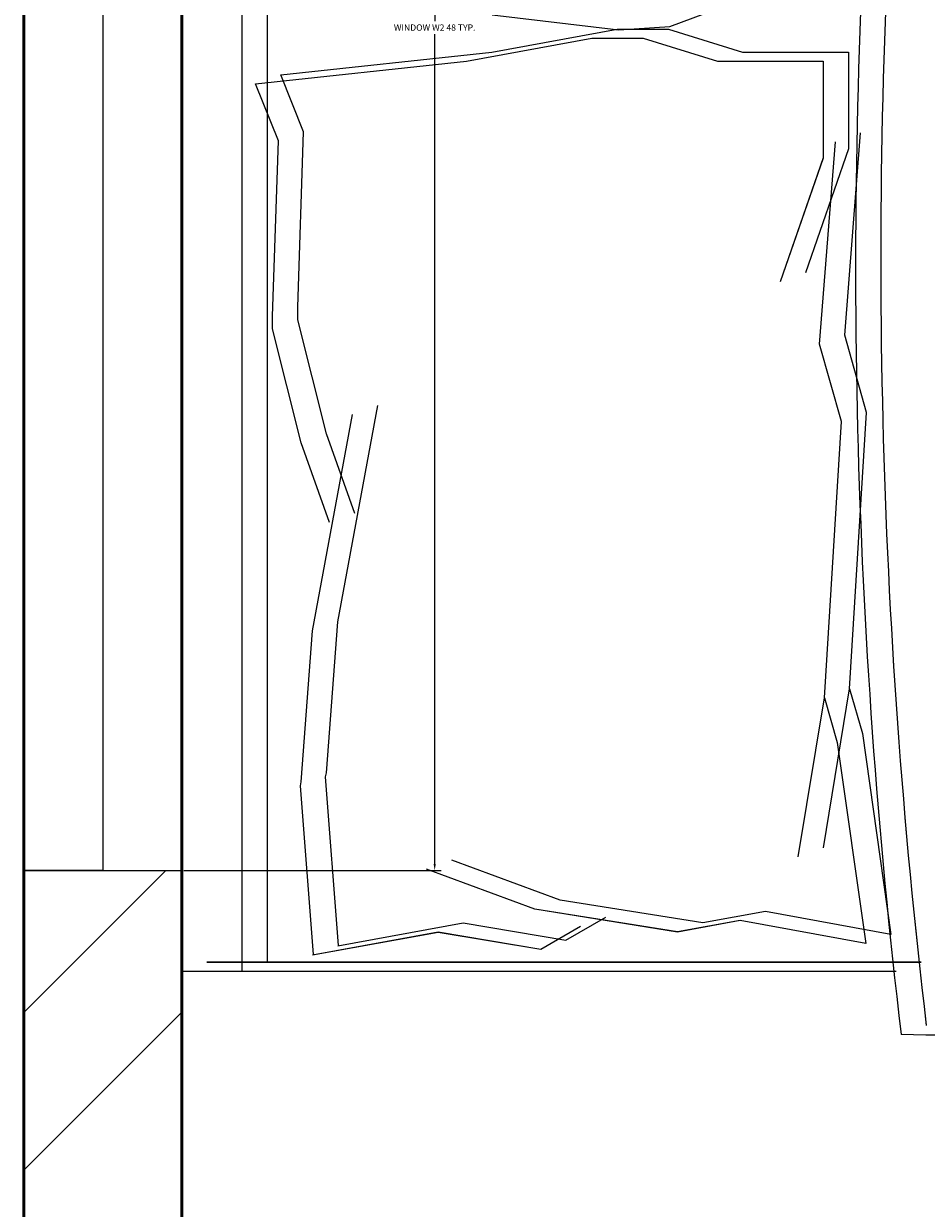
# Model space of a CAD drawing. Units: inches. Extents: x 1901 to 2863, y 888 to 2433.
# Tile 55 of 91: x 2025 to 2051, y 2127 to 2161. Entities that reach past the tile are written whole.
import ezdxf

# ---------------------------------------------------------------- set-up
doc = ezdxf.new("R2010")
doc.units = ezdxf.units.IN
for name, color, linetype, lineweight in [('A-ANNO-DIMS', 2, 'Continuous', 18), ('A-FURN', 8, 'Continuous', 18), ('A-GLAZ', 3, 'Continuous', 25), ('A-WALL', 7, 'Continuous', 50), ('A-WALL-PATT', 8, 'Continuous', 13)]:
    doc.layers.add(name, color=color, linetype=linetype, lineweight=lineweight)
doc.styles.get("Standard").update_dxf_attribs({"font": 'arial.ttf'})
doc.dimstyles.get("Standard").update_dxf_attribs({"dimtxt": 0.18, "dimasz": 0.18, "dimexe": 0.18, "dimexo": 0.0625, "dimgap": 0.09, "dimtad": 0, "dimtih": 1, "dimtoh": 1, "dimdec": 4, "dimzin": 0, "dimdsep": 46, "dimtxsty": 'Standard', "dimcen": 0.09, "dimadec": 0, "dimazin": 0, "dimtfac": 1, "dimtdec": 4, "dimtofl": 0, "dimtmove": 0, "dimatfit": 3, "dimfxl": 1, "dimtolj": 1, "dimtzin": 0, "dimarcsym": 0})

# ---------------------------------------------------------------- blocks, each defined once
blk = doc.blocks.new('BED-DOUBLE')
for p, q in [((0.026, 57.778), (0.026, 4.122)), ((13.922, 30.767), (15.988, 31.547)), ((13.922, 30.767), (15.988, 31.547)), ((8.859, 31.101), (12.464, 30.676)), ((8.859, 31.101), (12.464, 30.676)), ((12.464, 30.676), (13.922, 30.767)), ((12.464, 30.676), (13.922, 30.767)), ((8.132, 29.785), (11.704, 30.434)), ((8.132, 29.784), (11.704, 30.434)), ((8.85, 30.041), (12.422, 30.69)), ((8.85, 30.041), (12.422, 30.69)), ((11.704, 30.434), (13.165, 30.434)), ((11.704, 30.434), (13.165, 30.434)), ((12.422, 30.69), (13.883, 30.69)), ((12.422, 30.69), (13.883, 30.69)), ((13.165, 30.434), (15.275, 29.785)), ((13.165, 30.434), (15.275, 29.784)), ((13.883, 30.69), (15.993, 30.041)), ((13.883, 30.69), (15.993, 30.041)), ((2.844, 29.392), (8.85, 30.041)), ((2.844, 29.392), (8.85, 30.041)), ((15.993, 30.041), (19.003, 30.041)), ((15.993, 30.041), (19.003, 30.041)), ((19.003, 30.041), (19.003, 27.282)), ((19.003, 30.041), (19.003, 27.282)), ((2.126, 29.136), (8.132, 29.785)), ((2.126, 29.135), (8.132, 29.784)), ((15.275, 29.785), (18.286, 29.785)), ((15.275, 29.784), (18.286, 29.784)), ((18.286, 29.785), (18.286, 27.026)), ((18.286, 29.784), (18.286, 27.025)), ((3.493, 27.769), (2.844, 29.392)), ((3.493, 27.769), (2.844, 29.392)), ((2.775, 27.513), (2.126, 29.136)), ((2.775, 27.512), (2.126, 29.135)), ((3.331, 22.777), (3.493, 27.769)), ((3.331, 22.778), (3.493, 27.769)), ((18.898, 21.983), (19.351, 27.745)), ((18.898, 21.983), (19.351, 27.745)), ((2.613, 22.521), (2.775, 27.513)), ((2.613, 22.521), (2.775, 27.512)), ((18.18, 21.727), (18.633, 27.489)), ((18.18, 21.727), (18.633, 27.488)), ((18.286, 27.026), (17.061, 23.495)), ((18.286, 27.025), (17.061, 23.495)), ((19.003, 27.282), (17.779, 23.752)), ((19.003, 27.282), (17.779, 23.751)), ((3.331, 22.417), (3.331, 22.778)), ((3.331, 22.416), (3.331, 22.777)), ((2.613, 22.16), (2.613, 22.521)), ((2.613, 22.16), (2.613, 22.521)), ((4.142, 19.171), (3.331, 22.417)), ((4.142, 19.17), (3.331, 22.416)), ((3.425, 18.914), (2.613, 22.16)), ((3.425, 18.914), (2.613, 22.16)), ((19.523, 19.782), (18.898, 21.983)), ((19.523, 19.782), (18.898, 21.983)), ((18.806, 19.526), (18.18, 21.727)), ((18.806, 19.526), (18.18, 21.727)), ((4.467, 13.815), (5.603, 19.982)), ((4.467, 13.814), (5.603, 19.982)), ((3.749, 13.558), (4.886, 19.726)), ((3.749, 13.558), (4.886, 19.725)), ((19.039, 11.912), (19.523, 19.782)), ((19.039, 11.912), (19.523, 19.782)), ((18.322, 11.656), (18.806, 19.526)), ((18.322, 11.655), (18.806, 19.526)), ((4.236, 16.642), (3.425, 18.914)), ((4.236, 16.642), (3.425, 18.914)), ((4.954, 16.898), (4.142, 19.171)), ((4.954, 16.898), (4.142, 19.17)), ((3.425, 9.265), (3.749, 13.558)), ((3.425, 9.265), (3.749, 13.558)), ((4.142, 9.522), (4.467, 13.815)), ((4.142, 9.522), (4.467, 13.814)), ((18.291, 7.385), (19.039, 11.912)), ((18.291, 7.385), (19.039, 11.912)), ((19.039, 11.912), (19.402, 10.639)), ((19.039, 11.912), (19.402, 10.64)), ((17.573, 7.129), (18.322, 11.656)), ((17.573, 7.128), (18.322, 11.655)), ((18.322, 11.656), (18.684, 10.383)), ((18.322, 11.655), (18.684, 10.383)), ((19.402, 10.64), (20.214, 4.917)), ((19.402, 10.639), (20.214, 4.917)), ((18.684, 10.383), (19.496, 4.661)), ((18.684, 10.383), (19.496, 4.661)), ((4.122, 9.403), (4.142, 9.522)), ((4.122, 9.404), (4.142, 9.522)), ((3.404, 9.147), (3.425, 9.265)), ((3.404, 9.147), (3.425, 9.265)), ((3.774, 4.341), (3.404, 9.147)), ((3.774, 4.341), (3.404, 9.147)), ((4.492, 4.597), (4.122, 9.404)), ((4.492, 4.597), (4.122, 9.403)), ((10.08, 5.635), (6.996, 6.771)), ((10.08, 5.634), (6.996, 6.771)), ((10.798, 5.891), (7.714, 7.027)), ((10.798, 5.891), (7.714, 7.027)), ((14.857, 5.242), (10.798, 5.891)), ((14.857, 5.242), (10.798, 5.891)), ((14.139, 4.986), (10.08, 5.635)), ((14.139, 4.985), (10.08, 5.634)), ((10.961, 4.755), (12.097, 5.404)), ((10.961, 4.755), (12.097, 5.404)), ((16.642, 5.567), (14.857, 5.242)), ((16.642, 5.566), (14.857, 5.242)), ((20.214, 4.917), (16.642, 5.567)), ((20.214, 4.917), (16.642, 5.566)), ((4.467, 4.592), (8.039, 5.242)), ((4.467, 4.593), (8.038, 5.242)), ((8.038, 5.242), (10.961, 4.755)), ((8.039, 5.242), (10.961, 4.755)), ((10.243, 4.498), (11.379, 5.148)), ((10.243, 4.499), (11.379, 5.148)), ((15.925, 5.31), (14.139, 4.985)), ((15.924, 5.31), (14.139, 4.986)), ((19.496, 4.661), (15.924, 5.31)), ((19.496, 4.661), (15.925, 5.31)), ((3.749, 4.336), (7.321, 4.986)), ((3.749, 4.336), (7.321, 4.985)), ((7.321, 4.986), (10.243, 4.499)), ((7.321, 4.985), (10.243, 4.498))]:
    blk.add_line(p, q)
for centre, radius, start, end in [((205.143, 24.201), 185.219, 176.08655, 186.78213), ((205.143, 24.2), 185.219, 176.08655, 186.78213), ((204.426, 23.944), 185.219, 176.08655, 186.78213), ((204.426, 23.944), 185.219, 176.08655, 186.78213), ((22.589, 95.579), 93.531, 268.72178, 275.60397), ((22.589, 95.579), 93.531, 268.72178, 275.60397)]:
    blk.add_arc(centre, radius, start, end)
blk = doc.blocks.new('WIN-48')
for p, q in [((0, 2.25), (0, 4.5)), ((0, 4.5), (0, 0)), ((48, 2.25), (0, 2.25))]:
    blk.add_line(p, q)
blk = doc.blocks.new('*D21')
at = {"layer": 'A-ANNO-DIMS', "color": 0, "lineweight": -2, "transparency": 16777216}
for p, q in [((2029.489, 2184.739), (2036.806, 2184.739)), ((2036.626, 2184.559), (2036.626, 2160.923)), ((2036.626, 2136.919), (2036.626, 2160.556)), ((2029.489, 2136.739), (2036.806, 2136.739))]:
    blk.add_line(p, q, dxfattribs=at)
at = {"layer": 'A-ANNO-DIMS', "color": 0, "transparency": 16777216}
for points in [[(2036.596, 2184.559), (2036.656, 2184.559), (2036.626, 2184.739)], [(2036.596, 2136.919), (2036.656, 2136.919), (2036.626, 2136.739)]]:
    blk.add_solid(points, dxfattribs=at)
at = {"layer": 'Defpoints', "color": 0, "transparency": 16777216}
for p in [(2029.426, 2184.739), (2036.626, 2184.739), (2029.426, 2136.739)]:
    blk.add_point(p, dxfattribs=at)
at = {"layer": 'A-ANNO-DIMS', "color": 0, "transparency": 16777216, "insert": (2036.626, 2160.739), "char_height": 0.18, "attachment_point": 5}
blk.add_mtext('\\A1;WINDOW W2 48 TYP.', dxfattribs=at)

msp = doc.modelspace()

# ---------------------------------------------------------------- hatches: boundary and pattern name
at = {"layer": 'A-WALL-PATT'}
h = msp.add_hatch(dxfattribs=at)
h.set_pattern_fill('ANSI32', color=256)
h.paths.add_polyline_path([(2192.501, 2274.134), (2141.264, 2274.134), (2141.264, 2269.634), (2192.501, 2269.634)])
h.paths.add_polyline_path([(2259.926, 2274.134), (2216.501, 2274.134), (2216.501, 2269.634), (2255.426, 2269.634), (2255.426, 2214.634), (2250.809, 2214.634), (2250.809, 2210.134), (2259.926, 2210.134), (2259.926, 2215.134), (2271.756, 2215.134), (2271.756, 2217.384), (2271.756, 2219.634), (2259.926, 2219.634)])
h.paths.add_polyline_path([(2171.426, 2269.634), (2166.926, 2269.634), (2166.926, 2219.634), (2121.238, 2219.634), (2121.238, 2215.134), (2166.926, 2215.134), (2166.926, 2083.134), (2161.807, 2083.134), (2161.807, 2078.634), (2171.426, 2078.634), (2176.996, 2078.634), (2176.996, 2080.884), (2176.996, 2083.134), (2171.426, 2083.134), (2171.426, 2210.134), (2230.912, 2210.134), (2230.912, 2212.384), (2230.912, 2214.634), (2171.426, 2214.634)])
h.paths.add_polyline_path([(2117.264, 2274.134), (2089.426, 2274.134), (2089.426, 2219.634), (2081.136, 2219.634), (2081.136, 2215.134), (2089.426, 2215.134), (2098.004, 2215.134), (2098.004, 2217.384), (2098.004, 2219.634), (2093.926, 2219.634), (2093.926, 2269.634), (2117.264, 2269.634), (2117.264, 2271.884)])
h.paths.add_polyline_path([(2343.426, 2219.634), (2329.295, 2219.634), (2329.295, 2215.134), (2338.926, 2215.134), (2338.926, 2184.739), (2343.426, 2184.739)])
h.paths.add_polyline_path([(2338.926, 2083.134), (2329.295, 2083.134), (2208.966, 2083.134), (2208.966, 2078.634), (2338.926, 2078.634)])
h.paths.add_polyline_path([(2343.426, 2136.739), (2338.926, 2136.739), (2338.926, 1872.634), (2343.426, 1872.634)])
h.paths.add_polyline_path([(2343.426, 1863.634), (2397.68, 1863.634), (2397.68, 1821.634), (2384.138, 1821.634), (2384.138, 1812.634), (2418.33, 1812.634), (2418.33, 1817.134), (2418.33, 1821.634), (2406.68, 1821.634), (2406.68, 1863.634), (2459.499, 1863.634), (2459.499, 1821.634), (2447.138, 1821.634), (2447.138, 1812.634), (2459.499, 1812.634), (2468.499, 1812.634), (2468.499, 1872.634), (2394.426, 1872.634), (2334.426, 1872.634), (2334.426, 1812.634), (2343.426, 1812.634), (2353.251, 1812.634), (2353.251, 1821.634), (2343.426, 1821.634)])
h.paths.add_polyline_path([(2510.014, 1872.634), (2468.499, 1872.634), (2468.499, 1868.134), (2510.014, 1868.134)])
h.paths.add_polyline_path([(2514.009, 1817.134), (2468.499, 1817.134), (2468.499, 1812.634), (2482.114, 1812.634), (2482.114, 1800.606), (2486.614, 1800.606), (2486.614, 1812.634), (2514.009, 1812.634)])
h.paths.add_polyline_path([(2299.247, 1814.884), (2299.247, 1817.134), (2295.926, 1817.134), (2295.926, 1854.169), (2293.676, 1854.169), (2291.426, 1854.169), (2291.426, 1817.134), (2266.109, 1817.134), (2266.109, 1812.634), (2299.247, 1812.634)])
h.paths.add_polyline_path([(2218.109, 1817.134), (2206.46, 1817.134), (2171.426, 1817.134), (2171.426, 1949.134), (2190.1, 1949.134), (2190.1, 1953.634), (2163.468, 1953.634), (2163.468, 1949.134), (2166.926, 1949.134), (2166.926, 1817.134), (2114.297, 1817.134), (2114.297, 1812.634), (2218.109, 1812.634)])
h.paths.add_polyline_path([(2029.426, 1970.922), (2024.926, 1970.922), (2024.926, 1912.717), (2029.426, 1912.717)])
h.paths.add_polyline_path([(2132.297, 1953.634), (2113.926, 1953.634), (2113.926, 1975.888), (2111.676, 1975.888), (2109.426, 1975.888), (2109.426, 1953.634), (2029.426, 1953.634), (2029.426, 1949.134), (2132.297, 1949.134)])
h.paths.add_polyline_path([(2029.426, 1853.606), (2029.31, 1853.606), (2029.31, 1853.606), (2029.426, 1853.606), (2029.426, 1864.717), (2024.926, 1864.717), (2024.926, 1812.634), (2066.297, 1812.634), (2066.297, 1814.884), (2066.297, 1817.134), (2029.426, 1817.134)])
h.paths.add_polyline_path([(2122.926, 2010.088), (2120.676, 2010.088), (2118.426, 2010.088), (2118.426, 2006.134), (2029.426, 2006.134), (2029.426, 2001.634), (2109.426, 2001.634), (2109.426, 1998.041), (2113.926, 1998.041), (2113.926, 2001.634), (2122.926, 2001.634)])
h.paths.add_polyline_path([(2029.426, 2031.376), (2024.926, 2031.376), (2024.926, 1994.922), (2027.176, 1994.922), (2029.426, 1994.922)])
h.paths.add_polyline_path([(2029.426, 2136.739), (2024.926, 2136.739), (2024.926, 2067.376), (2027.176, 2067.376), (2029.426, 2067.376)])
h.paths.add_polyline_path([(2125.618, 2083.134), (2029.426, 2083.134), (2029.426, 2078.634), (2118.426, 2078.634), (2118.426, 2030.715), (2122.926, 2030.715), (2122.926, 2078.634), (2125.618, 2078.634)])
h.paths.add_polyline_path([(2029.426, 2215.134), (2040.468, 2215.134), (2040.468, 2217.384), (2040.468, 2219.634), (2024.926, 2219.634), (2024.926, 2184.739), (2029.426, 2184.739), (2029.426, 2187.778)])
h.paths.add_polyline_path([(2686.426, 2274.134), (2659.284, 2274.134), (2659.284, 2269.634), (2681.926, 2269.634), (2681.926, 2219.634), (2676.816, 2219.634), (2676.816, 2215.134), (2681.926, 2215.134), (2697.011, 2215.134), (2697.011, 2217.384), (2697.011, 2219.634), (2686.426, 2219.634)])
h.paths.add_polyline_path([(2609.926, 2269.634), (2635.284, 2269.634), (2635.284, 2274.134), (2571.431, 2274.134), (2571.431, 2269.634), (2605.426, 2269.634), (2605.426, 2214.634), (2549.098, 2214.634), (2549.098, 2210.134), (2605.426, 2210.134), (2605.426, 2083.134), (2601.014, 2083.134), (2601.014, 2080.884), (2601.014, 2078.634), (2609.926, 2078.634), (2616.162, 2078.634), (2616.162, 2080.884), (2616.162, 2083.134), (2609.926, 2083.134), (2609.926, 2215.134), (2651.465, 2215.134), (2651.465, 2217.384), (2651.465, 2219.634), (2609.926, 2219.634)])
h.paths.add_polyline_path([(2521.426, 2269.634), (2547.431, 2269.634), (2547.431, 2271.884), (2547.431, 2274.134), (2516.926, 2274.134), (2516.926, 2219.634), (2506.41, 2219.634), (2506.41, 2215.134), (2516.926, 2215.134), (2516.926, 2210.134), (2525.402, 2210.134), (2525.402, 2212.384), (2525.402, 2214.634), (2521.426, 2214.634)])
h.paths.add_polyline_path([(2456.011, 2219.634), (2439.426, 2219.634), (2439.426, 2187.888), (2443.926, 2187.888), (2443.926, 2215.134), (2456.011, 2215.134)])
h.paths.add_polyline_path([(2752.926, 2219.634), (2739.485, 2219.634), (2739.485, 2215.134), (2748.426, 2215.134), (2748.426, 2187.888), (2752.926, 2187.888)])
h.paths.add_polyline_path([(2752.926, 2139.888), (2748.426, 2139.888), (2748.426, 2083.134), (2648.416, 2083.134), (2648.416, 2078.634), (2654.926, 2078.634), (2654.926, 2039.437), (2659.426, 2039.437), (2659.426, 2078.634), (2748.426, 2078.634), (2748.426, 2063.429), (2752.926, 2063.429)])
h.paths.add_polyline_path([(2752.926, 2010.634), (2659.426, 2010.634), (2659.426, 2015.652), (2654.926, 2015.652), (2654.926, 2010.634), (2605.426, 2010.634), (2605.426, 1920.967), (2609.926, 1920.967), (2609.926, 2006.134), (2748.426, 2006.134), (2748.426, 1982.466), (2752.926, 1982.466)])
h.paths.add_polyline_path([(2752.926, 2027.429), (2748.426, 2027.429), (2748.426, 2010.634), (2752.926, 2010.634)])
h.paths.add_polyline_path([(2748.426, 1886.134), (2609.926, 1886.134), (2609.926, 1889.719), (2605.426, 1889.719), (2605.426, 1861.262), (2609.926, 1861.262), (2609.926, 1881.634), (2748.426, 1881.634)])
h.paths.add_polyline_path([(2456.855, 2228.831), (2498.401, 2228.831), (2498.401, 2247.488), (2456.855, 2247.488)], flags=9)
h.paths.add_polyline_path([(2038.602, 2237.418), (2080.174, 2237.418), (2080.174, 2256.075), (2038.602, 2256.075)], flags=9)
h.paths.add_polyline_path([(2292.009, 1062.394), (2539.932, 1062.394), (2539.932, 1099.487), (2292.009, 1099.487)], flags=9)
h.paths.add_polyline_path([(2424.91, 1832.253), (2448.513, 1832.253), (2448.513, 1846.678), (2424.91, 1846.678)], flags=25)
h.paths.add_polyline_path([(2359.076, 1832.253), (2382.678, 1832.253), (2382.678, 1846.678), (2359.076, 1846.678)], flags=25)
h.paths.add_polyline_path([(2352.899, 1684.802), (2367.543, 1684.802), (2367.543, 1697.167), (2352.899, 1697.167)], flags=9)
h.paths.add_polyline_path([(2079.288, 1755.826), (2169.024, 1755.826), (2169.024, 1774.372), (2079.288, 1774.372)], flags=9)
h.paths.add_polyline_path([(2404.09, 1373.857), (2404.09, 1463.593), (2385.544, 1463.593), (2385.544, 1373.857)], flags=9)
h.paths.add_polyline_path([(2268.091, 2236.371), (2309.636, 2236.371), (2309.636, 2255.028), (2268.091, 2255.028)], flags=9)
h.paths.add_polyline_path([(2575.96, 1700.951), (2665.696, 1700.951), (2665.696, 1719.498), (2575.96, 1719.498)], flags=9)
h.paths.add_polyline_path([(2302.962, 1878.474), (2329.524, 1878.474), (2329.524, 1888.777), (2302.962, 1888.777)], flags=9)
h.paths.add_polyline_path([(2097.415, 2240.576), (2126.573, 2240.576), (2126.573, 2259.233), (2097.415, 2259.233)], flags=9)
h.paths.add_polyline_path([(2208.725, 2246.124), (2237.882, 2246.124), (2237.882, 2264.781), (2208.725, 2264.781)], flags=9)
h.paths.add_polyline_path([(2038.147, 1925.958), (2076.987, 1925.958), (2076.987, 1944.615), (2038.147, 1944.615)], flags=9)
h.paths.add_polyline_path([(2239.144, 1926.672), (2288.465, 1926.672), (2288.465, 1945.329), (2239.144, 1945.329)], flags=9)
h.paths.add_polyline_path([(2175.429, 2007.33), (2212.356, 2007.33), (2212.356, 2025.987), (2175.429, 2025.987)], flags=9)
h.paths.add_polyline_path([(2225.034, 2091.794), (2263.875, 2091.794), (2263.875, 2110.451), (2225.034, 2110.451)], flags=9)
h.paths.add_polyline_path([(2035.398, 2098.478), (2074.238, 2098.478), (2074.238, 2117.135), (2035.398, 2117.135)], flags=9)
h.paths.add_polyline_path([(2050.102, 2029.209), (2083.26, 2029.209), (2083.26, 2047.866), (2050.102, 2047.866)], flags=9)
h.paths.add_polyline_path([(2069.677, 1956.719), (2098.835, 1956.719), (2098.835, 1975.376), (2069.677, 1975.376)], flags=25)
h.paths.add_polyline_path([(2328.62, 1753.336), (2361.663, 1753.336), (2361.663, 1771.993), (2328.62, 1771.993)], flags=9)
h.paths.add_polyline_path([(2395.162, 2060.888), (2395.162, 2140.654), (2378.676, 2140.654), (2378.676, 2060.888)], flags=9)
h.paths.add_polyline_path([(2463.728, 2059.02), (2492.886, 2059.02), (2492.886, 2077.677), (2463.728, 2077.677)], flags=9)
h.paths.add_polyline_path([(2458.027, 2181.536), (2496.868, 2181.536), (2496.868, 2200.194), (2458.027, 2200.194)], flags=9)
h.paths.add_polyline_path([(2527.577, 2243.074), (2556.735, 2243.074), (2556.735, 2261.731), (2527.577, 2261.731)], flags=9)
h.paths.add_polyline_path([(2694.461, 2232.767), (2736.033, 2232.767), (2736.033, 2251.425), (2694.461, 2251.425)], flags=9)
h.paths.add_polyline_path([(2637.821, 2249.225), (2666.979, 2249.225), (2666.979, 2267.882), (2637.821, 2267.882)], flags=9)
h.paths.add_polyline_path([(2623.687, 2183.541), (2662.528, 2183.541), (2662.528, 2202.199), (2623.687, 2202.199)], flags=9)
h.paths.add_polyline_path([(2691.965, 2021.5), (2725.124, 2021.5), (2725.124, 2040.157), (2691.965, 2040.157)], flags=9)
h.paths.add_polyline_path([(2621.043, 1975.912), (2662.335, 1975.912), (2662.335, 1994.569), (2621.043, 1994.569)], flags=25)
h.paths.add_polyline_path([(2479.032, 1927.62), (2519.844, 1927.62), (2519.844, 1946.277), (2479.032, 1946.277)], flags=9)
h.paths.add_polyline_path([(2670.941, 1849.076), (2716.005, 1849.076), (2716.005, 1867.734), (2670.941, 1867.734)], flags=9)
h.paths.add_polyline_path([(2523.613, 1782.956), (2550.175, 1782.956), (2550.175, 1793.26), (2523.613, 1793.26)], flags=9)
h.paths.add_polyline_path([(2450.841, 1207.331), (2492.386, 1207.331), (2492.386, 1225.989), (2450.841, 1225.989)], flags=9)
h.paths.add_polyline_path([(2527.751, 1203.841), (2556.908, 1203.841), (2556.908, 1222.499), (2527.751, 1222.499)], flags=9)
h.paths.add_polyline_path([(2639.111, 1207.2), (2668.268, 1207.2), (2668.268, 1225.857), (2639.111, 1225.857)], flags=9)
h.paths.add_polyline_path([(2692.594, 1218.965), (2734.167, 1218.965), (2734.167, 1237.623), (2692.594, 1237.623)], flags=9)
h.paths.add_polyline_path([(2669.266, 1366.329), (2708.106, 1366.329), (2708.106, 1384.987), (2669.266, 1384.987)], flags=9)
h.paths.add_polyline_path([(2463.313, 1358.031), (2502.153, 1358.031), (2502.153, 1376.688), (2463.313, 1376.688)], flags=9)
h.paths.add_polyline_path([(2494.725, 1449.963), (2531.652, 1449.963), (2531.652, 1468.62), (2494.725, 1468.62)], flags=9)
h.paths.add_polyline_path([(2675.565, 1422.157), (2708.724, 1422.157), (2708.724, 1440.815), (2675.565, 1440.815)], flags=9)
h.paths.add_polyline_path([(2685.634, 1493.891), (2714.792, 1493.891), (2714.792, 1512.548), (2685.634, 1512.548)], flags=9)
h.paths.add_polyline_path([(2686.805, 1529.913), (2725.645, 1529.913), (2725.645, 1548.57), (2686.805, 1548.57)], flags=9)
h.paths.add_polyline_path([(2503.651, 1537.991), (2552.972, 1537.991), (2552.972, 1556.648), (2503.651, 1556.648)], flags=9)
h.paths.add_polyline_path([(2291.713, 1643.504), (2318.275, 1643.504), (2318.275, 1653.807), (2291.713, 1653.807)], flags=9)
h.paths.add_polyline_path([(2450.626, 1610.52), (2477.189, 1610.52), (2477.189, 1620.824), (2450.626, 1620.824)], flags=9)
h.paths.add_polyline_path([(2359.985, 1551.814), (2422.253, 1551.814), (2422.253, 1562.117), (2359.985, 1562.117)], flags=9)
h.paths.add_polyline_path([(2280.106, 1249.006), (2321.651, 1249.006), (2321.651, 1267.663), (2280.106, 1267.663)], flags=9)
h.paths.add_polyline_path([(2164.057, 1274.232), (2193.215, 1274.232), (2193.215, 1292.889), (2164.057, 1292.889)], flags=9)
h.paths.add_polyline_path([(2118.21, 1277.694), (2151.252, 1277.694), (2151.252, 1296.351), (2118.21, 1296.351)], flags=9)
h.paths.add_polyline_path([(2031.946, 1268.529), (2073.519, 1268.529), (2073.519, 1287.187), (2031.946, 1287.187)], flags=9)
h.paths.add_polyline_path([(2050.199, 1409.079), (2089.04, 1409.079), (2089.04, 1427.736), (2050.199, 1427.736)], flags=9)
h.paths.add_polyline_path([(2243.743, 1421.032), (2282.584, 1421.032), (2282.584, 1439.689), (2243.743, 1439.689)], flags=9)
h.paths.add_polyline_path([(2190.746, 1509.769), (2231.558, 1509.769), (2231.558, 1528.426), (2190.746, 1528.426)], flags=9)
h.paths.add_polyline_path([(2058.392, 1475.415), (2091.55, 1475.415), (2091.55, 1494.073), (2058.392, 1494.073)], flags=9)
h.paths.add_polyline_path([(2062.447, 1553.09), (2091.605, 1553.09), (2091.605, 1571.747), (2062.447, 1571.747)], flags=9)
h.paths.add_polyline_path([(2219.524, 1590.365), (2266.147, 1590.365), (2266.147, 1609.022), (2219.524, 1609.022)], flags=9)
h.paths.add_polyline_path([(2041.072, 1584.188), (2079.912, 1584.188), (2079.912, 1602.845), (2041.072, 1602.845)], flags=9)

# ---------------------------------------------------------------- linework, layer by layer
at = {"layer": 'A-FURN'}
for p, q in [((2031.866, 2134.122), (2031.866, 2187.778)), ((2031.866, 2134.121), (2031.866, 2187.778)), ((2031.148, 2133.865), (2031.148, 2187.522)), ((2031.148, 2133.865), (2031.148, 2187.522)), ((2050.477, 2134.122), (2030.144, 2134.122)), ((2050.477, 2134.121), (2030.144, 2134.121)), ((2049.76, 2133.865), (2029.426, 2133.865)), ((2049.76, 2133.865), (2029.426, 2133.865))]:
    msp.add_line(p, q, dxfattribs=at)
at = {"layer": 'A-WALL'}
for p, q in [((2024.926, 2219.634), (2024.926, 1812.634)), ((2029.426, 2215.134), (2029.426, 1817.134))]:
    msp.add_line(p, q, dxfattribs=at)

# ---------------------------------------------------------------- block references
at = {"layer": 'A-FURN'}
msp.add_blockref('BED-DOUBLE', (2029.4, 2130), dxfattribs=at)
at = {"layer": 'A-GLAZ', "rotation": 90.00000000000097}
msp.add_blockref('WIN-48', (2029.426, 2136.74), dxfattribs=at)

# ---------------------------------------------------------------- dimensions: what is measured, and where the dimension line sits
at = {"layer": 'A-ANNO-DIMS'}
dim = msp.add_linear_dim(base=(2036.626, 2184.739), p1=(2029.426, 2136.739), p2=(2029.426, 2184.739), angle=90, text='WINDOW W2 <> TYP.', dimstyle='Standard', override={"dimdec": 0, "dimlfac": 1, "dimrnd": 0, "dimzin": 0, "dimdsep": 46, "dimlunit": 2}, dxfattribs=at)
dim.commit()
dim.dimension.update_dxf_attribs({"geometry": '*D21', "text_midpoint": (2036.626, 2160.739)})

doc.saveas('drawing.dxf')
